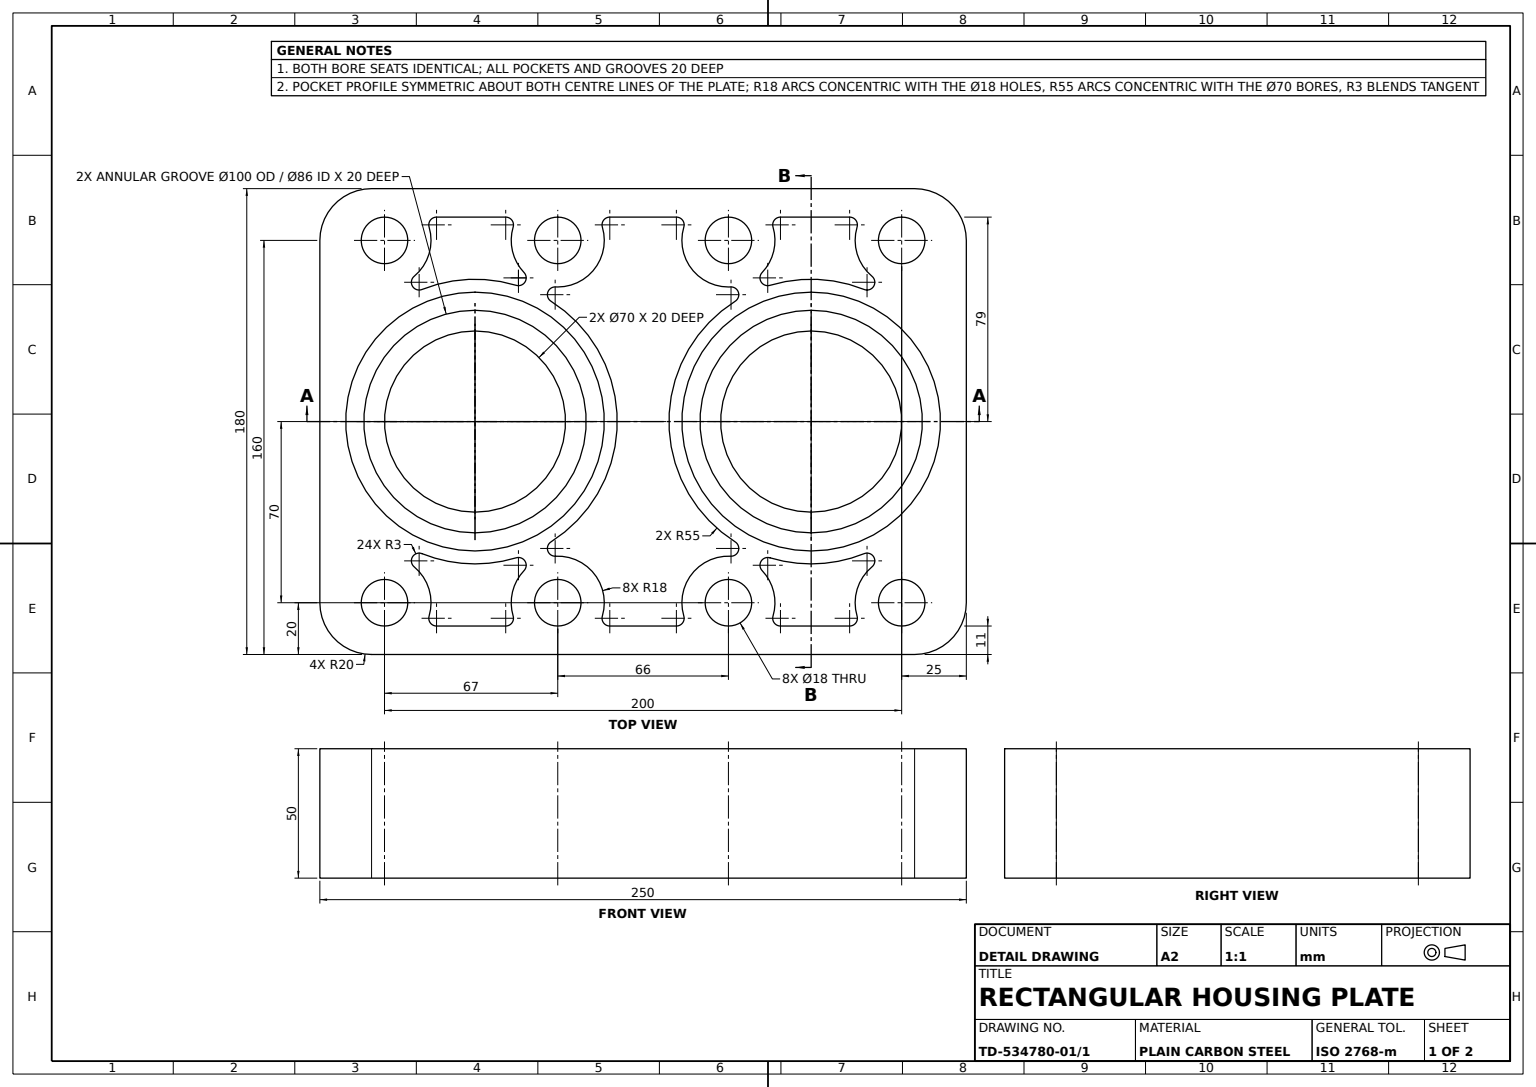
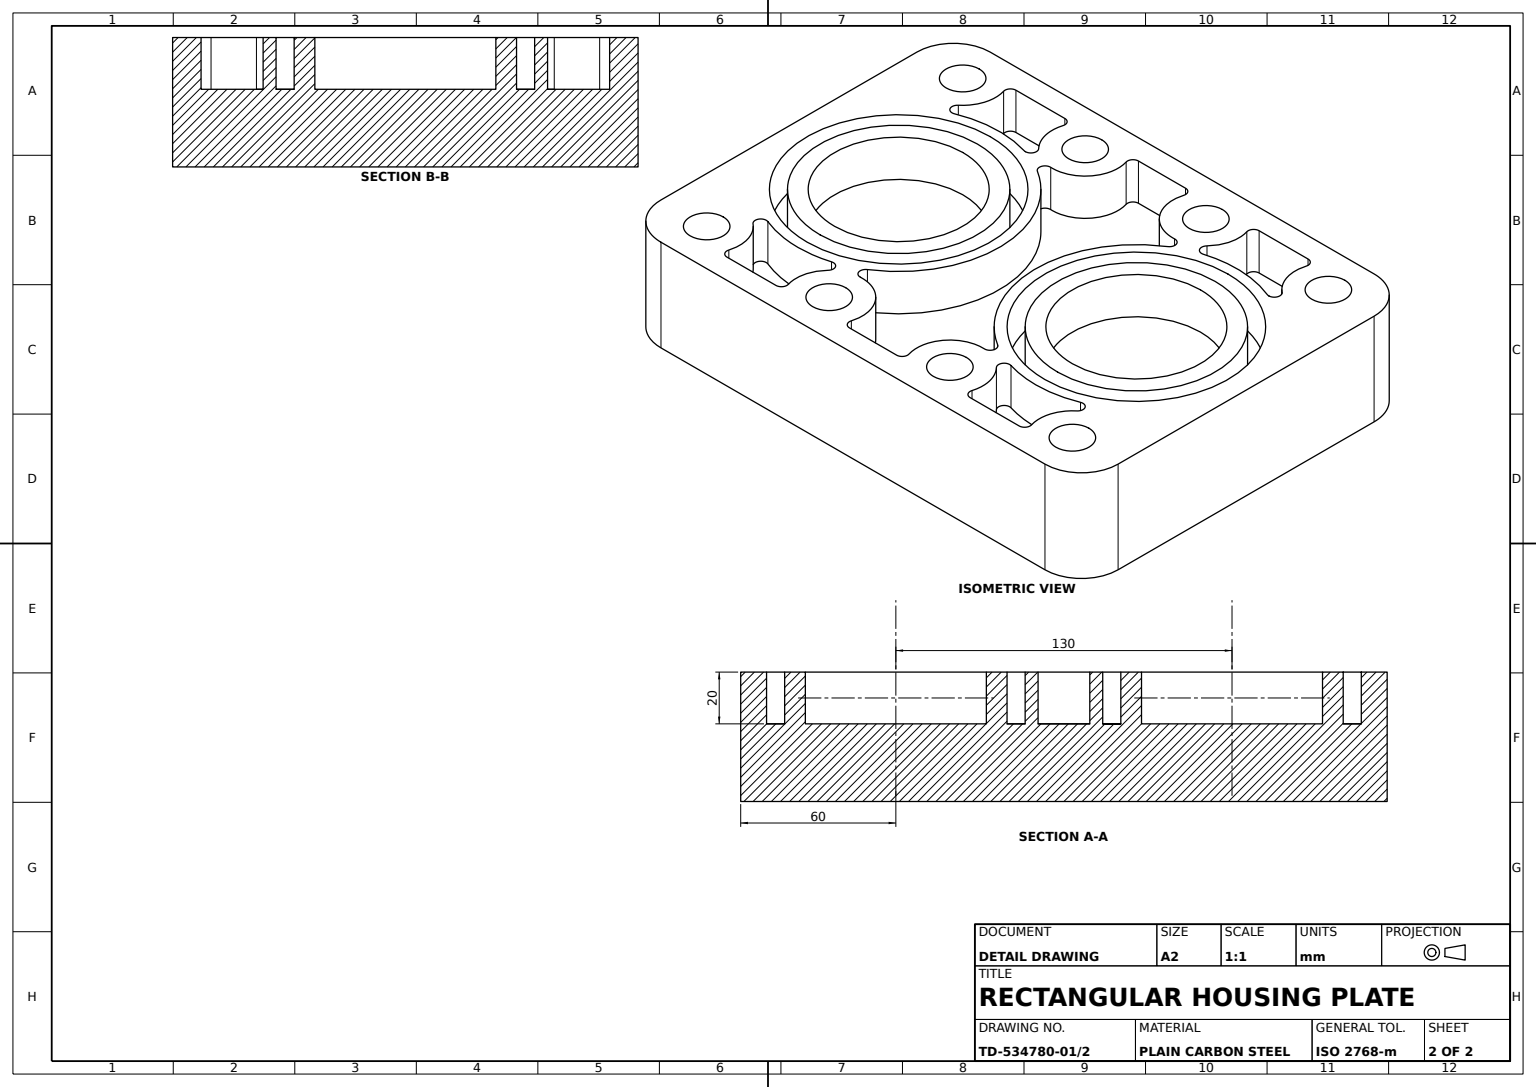
SolidWorks part; units mm, degrees
material "Plain Carbon Steel"
ref_plane "Front Plane" through (0, 0, 0) normal (0, 0, 1) x (1, 0, 0)
ref_plane "Top Plane" through (0, 0, 0) normal (0, 1, 0) x (1, 0, 0)
ref_plane "Right Plane" through (0, 0, 0) normal (1, 0, 0) x (0, 0, -1)
sketch "Base Plate Profile" plane through (0, 0, 0) normal (0, 1, 0) x (1, 0, 0)
  line L1 (125, 0) -> (125, 90)
  line L2 (125, 90) -> (-125, 90)
  line L3 (-125, 90) -> (-125, -90)
  line L4 (-125, -90) -> (125, -90)
  line L5 (125, -90) -> (125, 0)
  dimension "D1" = 250
  dimension "D2" = 180
  dimension "D3" = 125
  dimension "D4" = 90
extrude "Base Plate 250x180x50" add sketch "Base Plate Profile" along normal blind 50
sketch "Bore Seats and Pockets Profile" plane through (0, 50, 0) normal (0, 1, 0) x (1, 0, 0)
  line L2 (-53.1246, -79) -> (-79.8754, -79)
  line L3 (0, -79) -> (-12.8754, -79)
  line L4 (125, 90) -> (-125, 90) construction
  line L6 (0, 79) -> (12.8754, 79)
  line L7 (0, 79) -> (-12.8754, 79)
  line L9 (-53.1246, 79) -> (-79.8754, 79)
  line L10 (53.1246, 79) -> (79.8754, 79)
  line L11 (0, -79) -> (12.8754, -79)
  line L12 (53.1246, -79) -> (79.8754, -79)
  arc A0 (35.609, 46.4884) -> (35.609, -46.4884) centre (65, 0) ccw
  arc A1 (-85.4895, -51.041) -> (-49.0735, -52.6436) centre (-65, 0) ccw
  arc A2 (46.0327, 57.5843) -> (50.2497, 75.1429) centre (33, 70) ccw
  arc A3 (82.7503, 75.1429) -> (88.5203, 56.1357) centre (100, 70) ccw
  arc A4 (-46.0327, 57.5843) -> (-50.2497, 75.1429) centre (-33, 70) cw
  arc A5 (-82.7503, 75.1429) -> (-88.5203, 56.1357) centre (-100, 70) cw
  arc A10 (-88.5203, 56.1357) -> (-85.4895, 51.041) centre (-86.6071, 53.825) ccw
  arc A11 (-79.8754, 79) -> (-82.7503, 75.1429) centre (-79.8754, 76) ccw
  arc A12 (-50.2497, 75.1429) -> (-53.1246, 79) centre (-53.1246, 76) ccw
  arc A13 (-49.0735, 52.6436) -> (-46.0327, 57.5843) centre (-48.2048, 55.5151) ccw
  arc A14 (-33.8622, 52.0207) -> (-35.609, 46.4884) centre (-34.0058, 49.0241) ccw
  arc A15 (-12.8754, 79) -> (-15.7503, 75.1429) centre (-12.8754, 76) ccw
  arc A16 (15.7503, 75.1429) -> (12.8754, 79) centre (12.8754, 76) ccw
  arc A17 (35.609, 46.4884) -> (33.8622, 52.0207) centre (34.0058, 49.0241) ccw
  arc A18 (46.0327, 57.5843) -> (49.0735, 52.6436) centre (48.2048, 55.5151) ccw
  arc A19 (53.1246, 79) -> (50.2497, 75.1429) centre (53.1246, 76) ccw
  arc A20 (82.7503, 75.1429) -> (79.8754, 79) centre (79.8754, 76) ccw
  arc A21 (85.4895, 51.041) -> (88.5203, 56.1357) centre (86.6071, 53.825) ccw
  arc A22 (-15.7503, 75.1429) -> (-33.8622, 52.0207) centre (-33, 70) cw
  arc A23 (15.7503, 75.1429) -> (33.8622, 52.0207) centre (33, 70) ccw
  arc A24 (-88.5203, -56.1357) -> (-85.4895, -51.041) centre (-86.6071, -53.825) cw
  arc A25 (-82.7503, -75.1429) -> (-88.5203, -56.1357) centre (-100, -70) ccw
  arc A26 (-79.8754, -79) -> (-82.7503, -75.1429) centre (-79.8754, -76) cw
  arc A27 (-50.2497, -75.1429) -> (-53.1246, -79) centre (-53.1246, -76) cw
  arc A28 (-46.0327, -57.5843) -> (-50.2497, -75.1429) centre (-33, -70) ccw
  arc A29 (-49.0735, -52.6436) -> (-46.0327, -57.5843) centre (-48.2048, -55.5151) cw
  arc A30 (-33.8622, -52.0207) -> (-35.609, -46.4884) centre (-34.0058, -49.0241) cw
  arc A31 (-15.7503, -75.1429) -> (-33.8622, -52.0207) centre (-33, -70) ccw
  arc A32 (-12.8754, -79) -> (-15.7503, -75.1429) centre (-12.8754, -76) cw
  arc A33 (15.7503, -75.1429) -> (12.8754, -79) centre (12.8754, -76) cw
  arc A34 (15.7503, -75.1429) -> (33.8622, -52.0207) centre (33, -70) cw
  arc A35 (35.609, -46.4884) -> (33.8622, -52.0207) centre (34.0058, -49.0241) cw
  arc A36 (53.1246, -79) -> (50.2497, -75.1429) centre (53.1246, -76) cw
  arc A37 (46.0327, -57.5843) -> (50.2497, -75.1429) centre (33, -70) cw
  arc A38 (46.0327, -57.5843) -> (49.0735, -52.6436) centre (48.2048, -55.5151) cw
  arc A39 (85.4895, -51.041) -> (88.5203, -56.1357) centre (86.6071, -53.825) cw
  arc A40 (82.7503, -75.1429) -> (88.5203, -56.1357) centre (100, -70) cw
  arc A41 (82.7503, -75.1429) -> (79.8754, -79) centre (79.8754, -76) cw
  arc A42 (-49.0735, 52.6436) -> (-85.4895, 51.041) centre (-65, 0) ccw
  arc A43 (-35.609, -46.4884) -> (-35.609, 46.4884) centre (-65, 0) ccw
  arc A44 (85.4895, 51.041) -> (49.0735, 52.6436) centre (65, 0) ccw
  arc A45 (49.0735, -52.6436) -> (85.4895, -51.041) centre (65, 0) ccw
  circle A46 centre (-65, 0) radius 50
  circle A47 centre (65, 0) radius 50
  circle A48 centre (65, 0) radius 43
  circle A49 centre (-65, 0) radius 43
  circle A50 centre (65, 0) radius 35
  circle A51 centre (-65, 0) radius 35
  dimension "D1" = 36
  dimension "D2" = 110
  dimension "D3" = 3
  dimension "D5" = 110
  dimension "D7" = 70
  dimension "D11" = 70
  dimension "D13" = 36
  dimension "D16" = 36
  dimension "D17" = 36
  dimension "D19" = 79
  dimension "D9" = 100
  dimension "D10" = 86
  dimension "D4" = 65
  dimension "D6" = 65
  dimension "D8" = 35
  dimension "D12" = 70
  dimension "D14" = 67
  dimension "D15" = 66
  dimension "D18" = 67
  dimension "D25" = 11
  dimension "D26" = 79
extrude "Bore Seats and Pockets 20 Deep" cut sketch "Bore Seats and Pockets Profile" against normal blind 20 contours A44 A21 A3 A20 L10 A19 A2 A18 | A43 A30 A31 A32 L3 L11 A33 A34 A35 A0 A17 A23 A16 L6 L7 A15 A22 A14 | A42 A13 A4 A12 L9 A11 A5 A10 | A29 A1 A24 A25 A26 L2 A27 A28 | A45 A38 A37 A36 L12 A41 A40 A39 | A47 A48 | A50 | A46 A49 | A51
sketch "Bolt Holes Profile" plane through (0, 50, 0) normal (0, 1, 0) x (1, 0, 0)
  circle A0 centre (100, -70) radius 9
  circle A1 centre (33, -70) radius 9
  circle A2 centre (-33, -70) radius 9
  circle A3 centre (-100, -70) radius 9
  circle A4 centre (-100, 70) radius 9
  circle A5 centre (-33, 70) radius 9
  circle A6 centre (33, 70) radius 9
  circle A7 centre (100, 70) radius 9
  dimension "D1" = 18
  dimension "D2" = 18
  dimension "D3" = 18
  dimension "D4" = 18
  dimension "D5" = 18
  dimension "D6" = 18
  dimension "D7" = 18
  dimension "D8" = 18
extrude "Bolt Holes 8xØ18" cut sketch "Bolt Holes Profile" against normal blind 200
fillet "Corner Round R20 A" radius 20 1 edges at (-125, 25, 90)
fillet "Corner Round R20 B" radius 20 1 edges at (-125, 25, -90)
fillet "Corner Round R20 C" radius 20 1 edges at (125, 25, -90)
fillet "Corner Round R20 D" radius 20 1 edges at (125, 25, 90)
